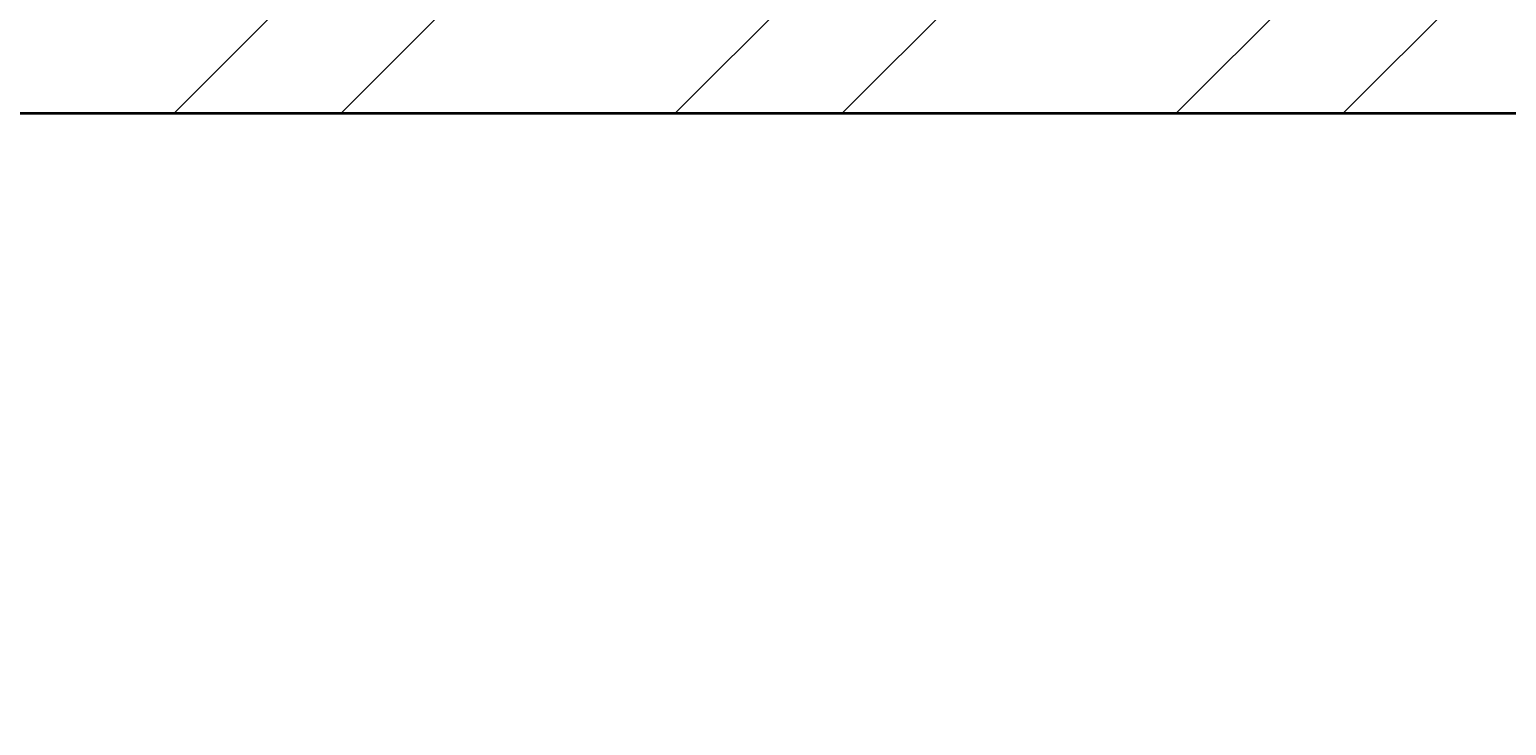
# Model space of a CAD drawing. Units: inches. Extents: x 1962 to 2771, y 1245 to 2660.
# Tile 55 of 114: x 2160 to 2200, y 2161 to 2180. Entities that reach past the tile are written whole.
import ezdxf

# ---------------------------------------------------------------- set-up
doc = ezdxf.new("R2010")
doc.units = ezdxf.units.IN
for name, color, linetype, lineweight in [('A-ANNO-DIMS', 2, 'Continuous', 18), ('A-WALL', 7, 'Continuous', 35), ('A-WALL-PATT', 252, 'Continuous', 13)]:
    doc.layers.add(name, color=color, linetype=linetype, lineweight=lineweight)
doc.styles.get("Standard").update_dxf_attribs({"font": 'arial.ttf'})
doc.dimstyles.get("Standard").update_dxf_attribs({"dimtxt": 0.18, "dimasz": 0.18, "dimexe": 0.18, "dimexo": 0.0625, "dimgap": 0.09, "dimtad": 0, "dimtih": 1, "dimtoh": 1, "dimdec": 4, "dimzin": 0, "dimdsep": 46, "dimtxsty": 'Standard', "dimcen": 0.09, "dimadec": 0, "dimazin": 0, "dimtfac": 1, "dimtdec": 4, "dimtofl": 0, "dimtmove": 0, "dimatfit": 3, "dimfxl": 1, "dimtolj": 1, "dimtzin": 0, "dimarcsym": 0})

# ---------------------------------------------------------------- blocks, each defined once
blk = doc.blocks.new('*D40')
at = {"layer": 'A-ANNO-DIMS', "color": 0, "lineweight": -2, "transparency": 16777216}
for p, q in [((2072.02, 2033.906), (2072.02, 2583.474)), ((2072.2, 2583.294), (2366.02, 2583.294)), ((2660.627, 2583.294), (2366.808, 2583.294)), ((2660.807, 2524.406), (2660.807, 2583.474))]:
    blk.add_line(p, q, dxfattribs=at)
at = {"layer": 'A-ANNO-DIMS', "color": 0, "transparency": 16777216}
for points in [[(2072.2, 2583.324), (2072.2, 2583.264), (2072.02, 2583.294)], [(2660.627, 2583.324), (2660.627, 2583.264), (2660.807, 2583.294)]]:
    blk.add_solid(points, dxfattribs=at)
at = {"layer": 'Defpoints', "color": 0, "transparency": 16777216}
for p in [(2660.807, 2583.294), (2660.807, 2524.344), (2072.02, 2033.844)]:
    blk.add_point(p, dxfattribs=at)
at = {"layer": 'A-ANNO-DIMS', "color": 0, "transparency": 16777216, "insert": (2366.414, 2583.294), "char_height": 0.18, "attachment_point": 5}
blk.add_mtext('\\A1;588.8', dxfattribs=at)

msp = doc.modelspace()

# ---------------------------------------------------------------- hatches: boundary and pattern name
at = {"layer": 'A-WALL-PATT'}
h = msp.add_hatch(dxfattribs=at)
h.set_pattern_fill('ANSI32', color=256)
h.paths.add_polyline_path([(2090.8074, 2467.3437), (2141.6481, 2467.3437), (2141.6481, 2469.5937), (2141.6481, 2471.8437), (2086.3074, 2471.8437), (2086.3074, 2422.5333), (2090.8074, 2422.5333)])
h.paths.add_polyline_path([(2282.7664, 2471.8437), (2204.8982, 2471.8437), (2204.8982, 2467.3437), (2234.8074, 2467.3437), (2234.8074, 2311.3437), (2228.7492, 2311.3437), (2228.7492, 2306.8437), (2234.8074, 2306.8437), (2331.9227, 2306.8437), (2331.9227, 2309.0937), (2331.9227, 2311.3437), (2239.3074, 2311.3437), (2239.3074, 2467.3437), (2282.7664, 2467.3437), (2282.7664, 2469.5937)])
h.paths.add_polyline_path([(2471.4531, 2519.8437), (2552.011, 2519.8437), (2564.3996, 2519.8437), (2564.3996, 2511.1389), (2568.8996, 2511.1389), (2568.8996, 2524.3437), (2466.9531, 2524.3437), (2466.9531, 2471.8437), (2450.0749, 2471.8437), (2446.4672, 2471.8437), (2446.4672, 2467.3437), (2450.0749, 2467.3437), (2475.9988, 2467.3437), (2475.9988, 2469.5937), (2475.9988, 2471.8437), (2471.4531, 2471.8437)])
h.paths.add_polyline_path([(2575.2231, 2469.5937), (2575.2231, 2471.8437), (2568.8996, 2471.8437), (2568.8996, 2487.1389), (2564.3996, 2487.1389), (2564.3996, 2471.8437), (2556.511, 2471.8437), (2499.2904, 2471.8437), (2499.2904, 2467.3437), (2507.8074, 2467.3437), (2507.8074, 2311.3437), (2414.863, 2311.3437), (2414.863, 2306.8437), (2512.3074, 2306.8437), (2517.0114, 2306.8437), (2517.0114, 2309.0937), (2517.0114, 2311.3437), (2512.3074, 2311.3437), (2512.3074, 2467.3437), (2575.2231, 2467.3437)])
h.paths.add_polyline_path([(2660.8074, 2471.8437), (2600.9602, 2471.8437), (2600.9602, 2467.3437), (2656.3074, 2467.3437), (2656.3074, 2432.5704), (2660.8074, 2432.5704)])
h.paths.add_polyline_path([(2660.8074, 2372.5704), (2656.3074, 2372.5704), (2656.3074, 2311.3437), (2600.276, 2311.3437), (2600.276, 2309.0937), (2600.276, 2306.8437), (2656.3074, 2306.8437), (2656.3074, 2296.2593), (2660.8074, 2296.2593)])
h.paths.add_polyline_path([(2572.3074, 2306.8437), (2577.1385, 2306.8437), (2577.1385, 2311.3437), (2551.082, 2311.3437), (2551.082, 2306.8437), (2567.8074, 2306.8437), (2567.8074, 2258.8437), (2540.0574, 2258.8437), (2540.0574, 2256.5937), (2540.0574, 2254.3437), (2567.8074, 2254.3437), (2656.3074, 2254.3437), (2656.3074, 2236.9085), (2660.8074, 2236.9085), (2660.8074, 2272.2593), (2656.3074, 2272.2593), (2656.3074, 2258.8437), (2572.3074, 2258.8437)])
h.paths.add_polyline_path([(2512.3074, 2254.3437), (2518.8716, 2254.3437), (2518.8716, 2256.5937), (2518.8716, 2258.8437), (2507.8074, 2258.8437), (2507.8074, 2177.8437), (2567.8074, 2177.8437), (2567.8074, 2172.9628), (2572.3074, 2172.9628), (2572.3074, 2177.8437), (2656.3074, 2177.8437), (2656.3074, 2166.4846), (2660.8074, 2166.4846), (2660.8074, 2200.9085), (2656.3074, 2200.9085), (2656.3074, 2182.3437), (2512.3074, 2182.3437)])
h.paths.add_polyline_path([(2656.3074, 2129.8437), (2572.3074, 2129.8437), (2572.3074, 2150.3044), (2570.0574, 2150.3044), (2567.8074, 2150.3044), (2567.8074, 2129.8437), (2507.8074, 2129.8437), (2507.8074, 2116.3027), (2510.0574, 2116.3027), (2512.3074, 2116.3027), (2512.3074, 2125.3437), (2567.8074, 2125.3437), (2572.3074, 2125.3437), (2656.3074, 2125.3437)])
h.paths.add_polyline_path([(2090.8074, 2362.5333), (2086.3074, 2362.5333), (2086.3074, 2298.6242), (2090.8074, 2298.6242), (2090.8074, 2306.8437), (2174.8074, 2306.8437), (2174.8074, 2286.4178), (2179.3074, 2286.4178), (2179.3074, 2306.8437), (2192.8641, 2306.8437), (2192.8641, 2309.0937), (2192.8641, 2311.3437), (2090.8074, 2311.3437)])
h.paths.add_polyline_path([(2209.156, 2258.8437), (2179.3074, 2258.8437), (2179.3074, 2263.2236), (2177.0574, 2263.2236), (2174.8074, 2263.2236), (2174.8074, 2258.8437), (2090.8074, 2258.8437), (2090.8074, 2274.6242), (2086.3074, 2274.6242), (2086.3074, 2238.2967), (2088.5574, 2238.2967), (2090.8074, 2238.2967), (2090.8074, 2254.3437), (2209.156, 2254.3437)])
h.paths.add_polyline_path([(2090.8074, 2177.8437), (2234.8074, 2177.8437), (2234.8074, 2173.1428), (2239.3074, 2173.1428), (2239.3074, 2258.8437), (2230.8442, 2258.8437), (2230.8442, 2256.5937), (2230.8442, 2254.3437), (2234.8074, 2254.3437), (2234.8074, 2182.3437), (2090.8074, 2182.3437), (2090.8074, 2202.2967), (2086.3074, 2202.2967), (2086.3074, 2140.0389), (2090.8074, 2140.0389)])
h.paths.add_polyline_path([(2090.8074, 2080.0389), (2086.3074, 2080.0389), (2086.3074, 2033.8437), (2090.8074, 2033.8437)], flags=17)
h.paths.add_polyline_path([(2244.9405, 2033.8437), (2239.3074, 2033.8437), (2239.3074, 2142.0665), (2237.2592, 2142.0665), (2234.8074, 2142.0665), (2234.8074, 2033.8437), (2090.8074, 2033.8437), (2076.5204, 2033.8437), (2072.0204, 2033.8437), (2072.0204, 2000.4493), (2076.5204, 2000.4493), (2076.5204, 2029.3437), (2090.8074, 2029.3437), (2244.9405, 2029.3437), (2244.9405, 2031.5937)])
h.paths.add_polyline_path([(2234.8074, 1933.3437), (2076.5204, 1933.3437), (2076.5204, 1952.4493), (2074.2704, 1952.4493), (2072.0204, 1952.4493), (2072.0204, 1933.3437), (2072.0204, 1928.8437), (2234.8074, 1928.8437)])
h.paths.add_polyline_path([(2090.8074, 1928.8437), (2086.3074, 1928.8437), (2086.3074, 1906.5013), (2090.8074, 1906.5013)])
h.paths.add_polyline_path([(2090.8074, 1846.5013), (2086.3074, 1846.5013), (2086.3074, 1769.9917), (2088.5574, 1769.9917), (2090.8074, 1769.9917), (2090.8074, 1780.3437), (2234.8074, 1780.3437), (2234.8074, 1708.3437), (2230.3764, 1708.3437), (2230.3764, 1703.8437), (2239.3074, 1703.8437), (2239.3074, 1792.6669), (2237.0574, 1792.6669), (2234.8074, 1792.6669), (2234.8074, 1784.8437), (2090.8074, 1784.8437)])
h.paths.add_polyline_path([(2239.3074, 1928.8437), (2244.9405, 1928.8437), (2244.9405, 1931.0937), (2244.9405, 1933.3437), (2234.8074, 1933.3437), (2234.8074, 1928.8437), (2234.8074, 1825.5949), (2239.3074, 1825.5949)])
h.paths.add_polyline_path([(2148.0425, 1649.0937), (2148.0425, 1651.3437), (2090.8074, 1651.3437), (2090.8074, 1646.8437), (2148.0425, 1646.8437)], flags=0)
h.paths.add_polyline_path([(2207.5601, 1708.3437), (2090.8074, 1708.3437), (2090.8074, 1703.8437), (2174.8074, 1703.8437), (2174.8074, 1651.3437), (2170.4457, 1651.3437), (2170.4457, 1646.8437), (2195.9924, 1646.8437), (2195.9924, 1649.0937), (2195.9924, 1651.3437), (2179.3074, 1651.3437), (2179.3074, 1703.8437), (2207.5601, 1703.8437), (2207.5601, 1706.0937)])
h.paths.add_polyline_path([(2090.8074, 1733.9917), (2086.3074, 1733.9917), (2086.3074, 1696.1032), (2088.5574, 1696.1032), (2090.8074, 1696.1032)])
h.paths.add_polyline_path([(2090.8074, 1672.1032), (2086.3074, 1672.1032), (2086.3074, 1600.3335), (2090.8074, 1600.3335)])
h.paths.add_polyline_path([(2090.8074, 1540.3335), (2086.3074, 1540.3335), (2086.3074, 1486.3437), (2139.6766, 1486.3437), (2139.6766, 1490.8437), (2090.8074, 1490.8437)])
h.paths.add_polyline_path([(2302.3876, 1490.8437), (2239.3074, 1490.8437), (2239.3074, 1646.8437), (2335.9994, 1646.8437), (2335.9994, 1651.3437), (2229.884, 1651.3437), (2229.884, 1646.8437), (2234.8074, 1646.8437), (2234.8074, 1490.8437), (2202.7103, 1490.8437), (2202.7103, 1488.5937), (2202.7103, 1486.3437), (2275.0699, 1486.3437), (2275.0699, 1475.772), (2279.5699, 1475.772), (2279.5699, 1486.3437), (2302.3876, 1486.3437)])
h.paths.add_polyline_path([(2279.5699, 1451.772), (2275.0699, 1451.772), (2275.0699, 1438.3437), (2174.8074, 1438.3437), (2174.8074, 1486.3437), (2179.7922, 1486.3437), (2179.7922, 1490.8437), (2163.3585, 1490.8437), (2163.3585, 1488.5937), (2163.3585, 1486.3437), (2170.3074, 1486.3437), (2170.3074, 1433.8437), (2279.5699, 1433.8437)])
h.paths.add_polyline_path([(2427.2363, 1490.8437), (2375.8074, 1490.8437), (2375.8074, 1646.8437), (2381.6401, 1646.8437), (2381.6401, 1651.3437), (2365.887, 1651.3437), (2365.887, 1649.0937), (2365.887, 1646.8437), (2371.3074, 1646.8437), (2371.3074, 1490.8437), (2327.5627, 1490.8437), (2327.5627, 1488.5937), (2327.5627, 1486.3437), (2371.3074, 1486.3437), (2371.3074, 1433.8437), (2375.8074, 1433.8437), (2375.8074, 1486.3437), (2427.2363, 1486.3437)])
h.paths.add_polyline_path([(2512.3074, 1646.8437), (2519.4351, 1646.8437), (2519.4351, 1649.0937), (2519.4351, 1651.3437), (2507.8074, 1651.3437), (2416.0063, 1651.3437), (2416.0063, 1649.0937), (2416.0063, 1646.8437), (2507.8074, 1646.8437), (2507.8074, 1490.8437), (2497.0532, 1490.8437), (2497.0532, 1488.5937), (2497.0532, 1486.3437), (2574.9344, 1486.3437), (2574.9344, 1476.0181), (2579.4344, 1476.0181), (2579.4344, 1486.3437), (2584.4872, 1486.3437), (2584.3074, 1490.8437), (2512.3074, 1490.8437)])
h.paths.add_polyline_path([(2470.5091, 1486.3437), (2473.9767, 1486.3437), (2473.9767, 1490.8437), (2449.6605, 1490.8437), (2449.6605, 1488.5937), (2449.6605, 1486.3437), (2466.0091, 1486.3437), (2466.0091, 1433.8437), (2470.5091, 1433.8437), (2579.4344, 1433.8437), (2579.4344, 1452.0181), (2574.9344, 1452.0181), (2574.9344, 1438.3437), (2554.5091, 1438.3437), (2470.5091, 1438.3437)])
h.paths.add_polyline_path([(2656.3074, 1490.8437), (2611.86, 1490.8437), (2611.86, 1486.3437), (2656.3074, 1486.3437)])
h.paths.add_polyline_path([(2660.8074, 1532.7007), (2658.5574, 1532.7007), (2656.3074, 1532.7007), (2656.3074, 1486.3437), (2660.8074, 1486.3437)])
h.paths.add_polyline_path([(2660.8074, 1664.9663), (2656.3074, 1664.9663), (2656.3074, 1651.3437), (2602.2313, 1651.3437), (2602.2313, 1646.8437), (2656.3074, 1646.8437), (2656.3074, 1592.7007), (2660.8074, 1592.7007)])
h.paths.add_polyline_path([(2660.8074, 1724.5221), (2656.3074, 1724.5221), (2656.3074, 1703.8437), (2542.4725, 1703.8437), (2542.4725, 1699.3437), (2567.8074, 1699.3437), (2567.8074, 1651.3437), (2552.7766, 1651.3437), (2552.7766, 1649.0937), (2552.7766, 1646.8437), (2577.2878, 1646.8437), (2577.2878, 1649.0937), (2577.2878, 1651.3437), (2572.3074, 1651.3437), (2572.3074, 1699.3437), (2656.3074, 1699.3437), (2656.3074, 1688.9663), (2660.8074, 1688.9663)])
h.paths.add_polyline_path([(2660.8074, 1880.6524), (2656.3074, 1880.6524), (2656.3074, 1832.8437), (2512.3074, 1832.8437), (2512.3074, 1837.8959), (2507.8074, 1837.8959), (2507.8074, 1828.3437), (2567.8074, 1828.3437), (2567.8074, 1804.3437), (2572.3074, 1804.3437), (2572.3074, 1828.3437), (2656.3074, 1828.3437), (2656.3074, 1818.6778), (2660.8074, 1818.6778)])
h.paths.add_polyline_path([(2660.8074, 1794.6778), (2656.3074, 1794.6778), (2656.3074, 1780.3437), (2572.3074, 1780.3437), (2572.3074, 1783.0303), (2570.0574, 1783.0303), (2567.8074, 1783.0303), (2567.8074, 1780.3437), (2507.8074, 1780.3437), (2507.8074, 1699.3437), (2517.8858, 1699.3437), (2517.8858, 1701.5937), (2517.8858, 1703.8437), (2512.3074, 1703.8437), (2512.3074, 1775.8437), (2656.3074, 1775.8437), (2656.3074, 1760.5221), (2660.8074, 1760.5221)])
h.paths.add_polyline_path([(2660.8074, 1981.3437), (2660.8074, 2020.2808), (2658.5574, 2020.2808), (2656.3074, 2020.2808), (2656.3074, 1981.3437), (2512.3074, 1981.3437), (2512.3074, 2086.6996), (2507.8074, 2086.6996), (2507.8074, 1981.3437), (2375.8074, 1981.3437), (2375.8074, 1986.8505), (2373.5574, 1986.8505), (2371.3074, 1986.8505), (2371.3074, 1973.2607), (2375.8074, 1973.2607), (2375.8074, 1976.8437), (2507.8074, 1976.8437), (2507.8074, 1865.4281), (2510.0574, 1865.4281), (2512.3074, 1865.4281), (2512.3074, 1976.8437), (2660.8074, 1976.8437)])
h.paths.add_polyline_path([(2375.8074, 1940.297), (2373.5574, 1940.297), (2371.3074, 1940.297), (2371.3074, 1933.3437), (2278.4434, 1933.3437), (2278.4434, 1928.8437), (2371.3074, 1928.8437), (2371.3074, 1651.3437), (2375.8074, 1651.3437)])
h.paths.add_polyline_path([(2660.8074, 1976.8437), (2656.3074, 1976.8437), (2656.3074, 1940.6524), (2660.8074, 1940.6524)], flags=17)
h.paths.add_polyline_path([(2660.8074, 2142.4846), (2656.3074, 2142.4846), (2656.3074, 2080.2808), (2660.8074, 2080.2808)])
h.paths.add_polyline_path([(2381.4189, 2311.3437), (2375.8074, 2311.3437), (2375.8074, 2467.3437), (2424.7242, 2467.3437), (2424.7242, 2469.5937), (2424.7242, 2471.8437), (2375.8074, 2471.8437), (2375.8074, 2524.3437), (2371.3074, 2524.3437), (2371.3074, 2471.8437), (2307.2097, 2471.8437), (2307.2097, 2467.3437), (2371.3074, 2467.3437), (2371.3074, 2311.3437), (2366.8901, 2311.3437), (2366.8901, 2306.8437), (2371.3074, 2306.8437), (2371.3074, 2033.8437), (2279.6589, 2033.8437), (2279.6589, 2029.3437), (2371.3074, 2029.3437), (2371.3074, 2014.2598), (2375.8074, 2014.2598), (2375.8074, 2306.8437), (2381.4189, 2306.8437)])
h.paths.add_polyline_path([(2263.3074, 2524.3437), (2170.3074, 2524.3437), (2170.3074, 2519.8437), (2170.3074, 2471.8437), (2165.0312, 2471.8437), (2165.0312, 2467.3437), (2179.6721, 2467.3437), (2179.6721, 2469.5161), (2179.6721, 2471.8437), (2174.8074, 2471.8437), (2174.8074, 2519.8437), (2258.8074, 2519.8437), (2258.8074, 2511.6436), (2263.3074, 2511.6436)])
h.paths.add_polyline_path([(2245.0232, 1361.4123), (2492.9468, 1361.4123), (2492.9468, 1398.505), (2245.0232, 1398.505)], flags=9)
h.paths.add_polyline_path([(2388.1434, 2086.6936), (2425.0704, 2086.6936), (2425.0704, 2105.3509), (2388.1434, 2105.3509)], flags=9)
h.paths.add_polyline_path([(2404.922, 2242.6744), (2445.7337, 2242.6744), (2445.7337, 2261.3318), (2404.922, 2261.3318)], flags=9)
h.paths.add_polyline_path([(2269.4107, 2156.7935), (2306.3378, 2156.7935), (2306.3378, 2175.4508), (2269.4107, 2175.4508)], flags=9)
h.paths.add_polyline_path([(2269.3277, 2233.4343), (2306.2547, 2233.4343), (2306.2547, 2252.0917), (2269.3277, 2252.0917)], flags=9)
h.paths.add_polyline_path([(2431.6052, 2320.6922), (2470.4456, 2320.6922), (2470.4456, 2339.3495), (2431.6052, 2339.3495)], flags=25)
h.paths.add_polyline_path([(2249.6902, 2315.7608), (2288.5306, 2315.7608), (2288.5306, 2334.4182), (2249.6902, 2334.4182)], flags=25)
h.paths.add_polyline_path([(2096.9301, 2314.3181), (2135.7704, 2314.3181), (2135.7704, 2332.9755), (2096.9301, 2332.9755)], flags=25)
h.paths.add_polyline_path([(2134.3475, 2285.7089), (2161.4655, 2285.7089), (2161.4655, 2304.3662), (2134.3475, 2304.3662)], flags=9)
h.paths.add_polyline_path([(2126.5155, 2209.4076), (2159.9227, 2209.4076), (2159.9227, 2228.065), (2126.5155, 2228.065)], flags=25)
h.paths.add_polyline_path([(2110.5753, 2141.5299), (2149.4157, 2141.5299), (2149.4157, 2160.1872), (2110.5753, 2160.1872)], flags=25)
h.paths.add_polyline_path([(2249.8618, 1968.3317), (2286.3966, 1968.3317), (2286.3966, 1986.989), (2249.8618, 1986.989)], flags=9)
h.paths.add_polyline_path([(2395.9507, 1777.0051), (2436.7624, 1777.0051), (2436.7624, 1795.6625), (2395.9507, 1795.6625)], flags=9)
h.paths.add_polyline_path([(2398.5259, 1888.5651), (2435.0062, 1888.5651), (2435.0062, 1907.2224), (2398.5259, 1907.2224)], flags=25)
h.paths.add_polyline_path([(2259.3506, 1728.3559), (2296.2776, 1728.3559), (2296.2776, 1747.0132), (2259.3506, 1747.0132)], flags=9)
h.paths.add_polyline_path([(2271.3698, 1845.268), (2308.2968, 1845.268), (2308.2968, 1863.9253), (2271.3698, 1863.9253)], flags=9)
h.paths.add_polyline_path([(2120.9355, 1786.3027), (2159.7759, 1786.3027), (2159.7759, 1804.9601), (2120.9355, 1804.9601)], flags=25)
h.paths.add_polyline_path([(2121.3164, 1732.1043), (2154.7236, 1732.1043), (2154.7236, 1750.7616), (2121.3164, 1750.7616)], flags=25)
h.paths.add_polyline_path([(2118.3706, 1678.8997), (2147.5282, 1678.8997), (2147.5282, 1697.557), (2118.3706, 1697.557)], flags=25)
h.paths.add_polyline_path([(2385.9227, 1493.557), (2424.763, 1493.557), (2424.763, 1512.2143), (2385.9227, 1512.2143)], flags=25)
h.paths.add_polyline_path([(2248.7058, 1500.0256), (2287.5462, 1500.0256), (2287.5462, 1518.6829), (2248.7058, 1518.6829)], flags=25)
h.paths.add_polyline_path([(2104.1669, 1617.3771), (2143.0073, 1617.3771), (2143.0073, 1636.0344), (2104.1669, 1636.0344)], flags=9)
h.paths.add_polyline_path([(2096.0714, 1447.8824), (2137.3845, 1447.8824), (2137.3845, 1458.1859), (2096.0714, 1458.1859)], flags=9)
h.paths.add_polyline_path([(2180.6114, 1440.325), (2209.7689, 1440.325), (2209.7689, 1458.9823), (2180.6114, 1458.9823)], flags=25)
h.paths.add_polyline_path([(2316.1698, 1447.9637), (2357.4829, 1447.9637), (2357.4829, 1458.2673), (2316.1698, 1458.2673)], flags=9)
h.paths.add_polyline_path([(2397.6187, 1447.9637), (2438.9318, 1447.9637), (2438.9318, 1458.2673), (2397.6187, 1458.2673)], flags=9)
h.paths.add_polyline_path([(2473.0778, 1439.5953), (2502.2354, 1439.5953), (2502.2354, 1458.2527), (2473.0778, 1458.2527)], flags=25)
h.paths.add_polyline_path([(2589.7027, 1447.8819), (2631.0158, 1447.8819), (2631.0158, 1458.1855), (2589.7027, 1458.1855)], flags=9)
h.paths.add_polyline_path([(2522.4009, 1497.5285), (2561.2413, 1497.5285), (2561.2413, 1516.1859), (2522.4009, 1516.1859)], flags=25)
h.paths.add_polyline_path([(2579.6565, 1671.3482), (2608.8141, 1671.3482), (2608.8141, 1690.0056), (2579.6565, 1690.0056)], flags=25)
h.paths.add_polyline_path([(2544.7038, 1725.5064), (2578.1111, 1725.5064), (2578.1111, 1744.1637), (2544.7038, 1744.1637)], flags=25)
h.paths.add_polyline_path([(2578.1191, 1807.472), (2607.2766, 1807.472), (2607.2766, 1826.1293), (2578.1191, 1826.1293)], flags=25)
h.paths.add_polyline_path([(2595.0614, 1835.1839), (2633.9018, 1835.1839), (2633.9018, 1853.8413), (2595.0614, 1853.8413)], flags=25)
h.paths.add_polyline_path([(2567.0097, 2097.7035), (2605.8501, 2097.7035), (2605.8501, 2116.3609), (2567.0097, 2116.3609)], flags=9)
h.paths.add_polyline_path([(2586.644, 2134.6454), (2615.8015, 2134.6454), (2615.8015, 2153.3027), (2586.644, 2153.3027)], flags=9)
h.paths.add_polyline_path([(2544.6185, 2212.6783), (2578.0258, 2212.6783), (2578.0258, 2231.3356), (2544.6185, 2231.3356)], flags=25)
h.paths.add_polyline_path([(2577.0273, 2256.9023), (2606.1849, 2256.9023), (2606.1849, 2275.5597), (2577.0273, 2275.5597)], flags=24)
h.paths.add_polyline_path([(2605.2683, 2315.2821), (2644.1087, 2315.2821), (2644.1087, 2333.9395), (2605.2683, 2333.9395)], flags=25)
h.paths.add_polyline_path([(2583.1244, 2496.1815), (2624.4375, 2496.1815), (2624.4375, 2506.4851), (2583.1244, 2506.4851)], flags=9)
h.paths.add_polyline_path([(2474.761, 2497.0823), (2503.9185, 2497.0823), (2503.9185, 2515.7397), (2474.761, 2515.7397)], flags=25)
h.paths.add_polyline_path([(2387.5787, 2494.2563), (2428.902, 2494.2563), (2428.902, 2504.5598), (2387.5787, 2504.5598)], flags=9)
h.paths.add_polyline_path([(2300.1657, 2500.1564), (2341.4788, 2500.1564), (2341.4788, 2510.46), (2300.1657, 2510.46)], flags=25)
h.paths.add_polyline_path([(2176.8589, 2497.5843), (2206.0165, 2497.5843), (2206.0165, 2516.2416), (2176.8589, 2516.2416)], flags=25)
h.paths.add_polyline_path([(2097.4668, 2494.9762), (2138.7799, 2494.9762), (2138.7799, 2505.2798), (2097.4668, 2505.2798)], flags=9)

# ---------------------------------------------------------------- linework, layer by layer
at = {"layer": 'A-WALL'}
msp.add_line((2090.8074, 2177.8437), (2234.8074, 2177.8437), dxfattribs=at)

# ---------------------------------------------------------------- dimensions: what is measured, and where the dimension line sits
at = {"layer": 'A-ANNO-DIMS'}
dim = msp.add_linear_dim(base=(2660.8074, 2583.2937), p1=(2072.0204, 2033.8437), p2=(2660.8074, 2524.3437), dimstyle='Standard', override={"dimdec": 1, "dimlfac": 1, "dimrnd": 0, "dimzin": 0, "dimdsep": 46, "dimlunit": 2}, dxfattribs=at)
dim.commit()
dim.dimension.update_dxf_attribs({"geometry": '*D40', "text_midpoint": (2366.4139, 2583.2937)})

doc.saveas('drawing.dxf')
